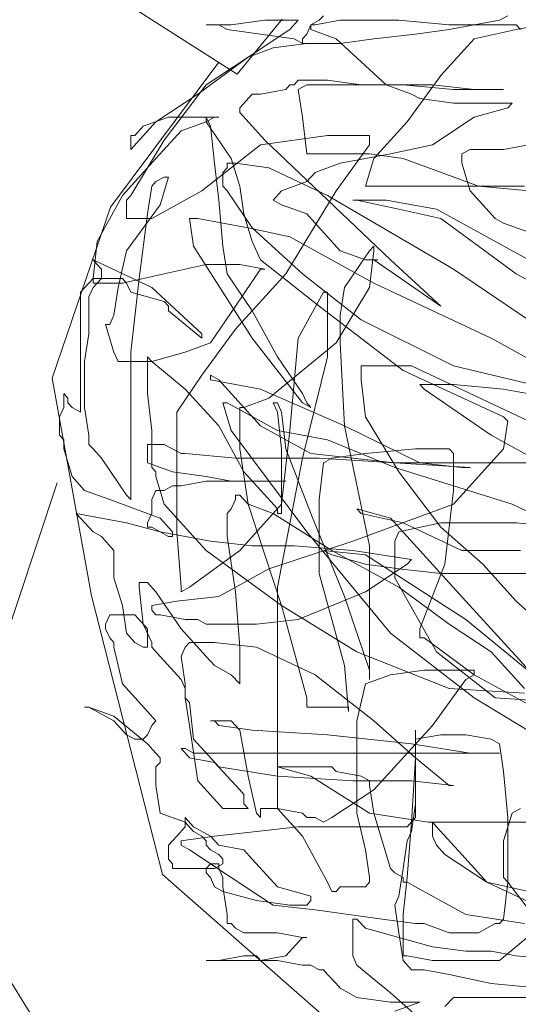
# Model space of a CAD drawing. Units: inches. Extents: x 1994 to 3075, y 3517 to 3950.
# Tile 40 of 58: x 1994.64257 to 1994.646332, y 3553.741889 to 3553.749313. Entities that reach past the tile are written whole.
import ezdxf

# ---------------------------------------------------------------- set-up
doc = ezdxf.new("R2010")
doc.units = ezdxf.units.IN
doc.layers.add('A-FURN-REFR', color=8, linetype='Continuous', lineweight=13)

msp = doc.modelspace()

# ---------------------------------------------------------------- linework, layer by layer
at = {"layer": 'A-FURN-REFR'}
for p, q in [((1994.6422829, 3553.7501317), (1994.644212, 3553.7489025)), ((1994.6444196, 3553.7493078), (1994.6441668, 3553.7492731)), ((1994.644212, 3553.7489025), (1994.644551, 3553.7493173)), ((1994.6446725, 3553.7493078), (1994.6444196, 3553.7493078)), ((1994.6446093, 3553.7492383), (1994.6446725, 3553.7493078)), ((1994.6448306, 3553.7493078), (1994.6447673, 3553.7492731)), ((1994.644799, 3553.7492731), (1994.6449886, 3553.7493078)), ((1994.6448622, 3553.7493426), (1994.6448306, 3553.7493078)), ((1994.6449886, 3553.7493078), (1994.6454312, 3553.7493078)), ((1994.6454312, 3553.7493078), (1994.6458105, 3553.7492731)), ((1994.6460001, 3553.7492731), (1994.6461898, 3553.7493078)), ((1994.6461898, 3553.7493078), (1994.646253, 3553.7493426)), ((1994.6439771, 3553.7492731), (1994.6440719, 3553.7492731)), ((1994.6441668, 3553.7492731), (1994.6439771, 3553.7492731)), ((1994.6440719, 3553.7492731), (1994.6441351, 3553.7492383)), ((1994.6441351, 3553.7492383), (1994.644388, 3553.7492037)), ((1994.6442932, 3553.7490299), (1994.6446093, 3553.7492383)), ((1994.6447673, 3553.7492731), (1994.6447357, 3553.7492037)), ((1994.6447673, 3553.7492731), (1994.644799, 3553.7492731)), ((1994.6447673, 3553.7492383), (1994.6447673, 3553.7492731)), ((1994.644957, 3553.7491689), (1994.6447673, 3553.7492383)), ((1994.6455576, 3553.7492037), (1994.6458105, 3553.7492383)), ((1994.6458105, 3553.7492731), (1994.6463162, 3553.7492731)), ((1994.6458105, 3553.7492383), (1994.6460001, 3553.7492731)), ((1994.6463162, 3553.7492383), (1994.6460001, 3553.7491689)), ((1994.6463162, 3553.7492731), (1994.6463478, 3553.7492383)), ((1994.6465059, 3553.7492731), (1994.6463162, 3553.7492383)), ((1994.644388, 3553.7492037), (1994.6446409, 3553.7491689)), ((1994.6446409, 3553.7491689), (1994.6447041, 3553.7491341)), ((1994.6447357, 3553.7492037), (1994.6447041, 3553.7491689)), ((1994.6447041, 3553.7491689), (1994.6447041, 3553.7491341)), ((1994.6453363, 3553.7488214), (1994.644957, 3553.7491689)), ((1994.6449886, 3553.7491341), (1994.6452415, 3553.7491689)), ((1994.6452415, 3553.7491689), (1994.6455576, 3553.7492037)), ((1994.6460001, 3553.7491689), (1994.6457472, 3553.7488909)), ((1994.6444829, 3553.7490994), (1994.6442932, 3553.7490299)), ((1994.6447357, 3553.7491341), (1994.6444829, 3553.7490994)), ((1994.6447041, 3553.7491341), (1994.6449886, 3553.7491341)), ((1994.6447041, 3553.7491341), (1994.6447357, 3553.7491341)), ((1994.6439139, 3553.7487519), (1994.6442932, 3553.7490299)), ((1994.6442932, 3553.7490299), (1994.6439771, 3553.7488214)), ((1994.6432553, 3553.7478986), (1994.6440722, 3553.7489916)), ((1994.6457472, 3553.7488909), (1994.6454944, 3553.7485434)), ((1994.6439771, 3553.7488214), (1994.643661, 3553.7484045)), ((1994.6445777, 3553.7487867), (1994.644388, 3553.7487519)), ((1994.6446093, 3553.7488214), (1994.6445777, 3553.7487867)), ((1994.6446409, 3553.7488214), (1994.6446093, 3553.7488214)), ((1994.6446725, 3553.7488562), (1994.6446409, 3553.7488214)), ((1994.6448938, 3553.7488562), (1994.6446725, 3553.7488562)), ((1994.6446725, 3553.7487867), (1994.6447357, 3553.7488214)), ((1994.6447041, 3553.7485782), (1994.6446725, 3553.7487867)), ((1994.6447357, 3553.7488214), (1994.645684, 3553.7488214)), ((1994.6451466, 3553.7488214), (1994.6448938, 3553.7488562)), ((1994.6454628, 3553.7488214), (1994.6451466, 3553.7488214)), ((1994.645526, 3553.7487519), (1994.6453363, 3553.7488214)), ((1994.6458421, 3553.7487867), (1994.6454628, 3553.7488214)), ((1994.645684, 3553.7488214), (1994.6460001, 3553.7487867)), ((1994.6462214, 3553.7487867), (1994.6458421, 3553.7487867)), ((1994.6460001, 3553.7487867), (1994.6462214, 3553.7487867)), ((1994.6435978, 3553.7485434), (1994.6439139, 3553.7487519)), ((1994.6443248, 3553.7487519), (1994.64423, 3553.7486477)), ((1994.644388, 3553.7487519), (1994.6443248, 3553.7487519)), ((1994.6455892, 3553.7487172), (1994.645526, 3553.7487519)), ((1994.6458421, 3553.7486824), (1994.6455892, 3553.7487172)), ((1994.64423, 3553.7486477), (1994.64423, 3553.7486129)), ((1994.6462846, 3553.7486824), (1994.6458421, 3553.7486824)), ((1994.6460001, 3553.7485782), (1994.646253, 3553.7486477)), ((1994.646253, 3553.7486477), (1994.6462846, 3553.7486824)), ((1994.6436926, 3553.7485782), (1994.6435029, 3553.7485087)), ((1994.6440719, 3553.7485782), (1994.6436926, 3553.7485782)), ((1994.6439771, 3553.7485782), (1994.6440087, 3553.7485087)), ((1994.6439771, 3553.7485434), (1994.6439771, 3553.7485782)), ((1994.6439771, 3553.7485434), (1994.6440403, 3553.7485782)), ((1994.6440403, 3553.7485782), (1994.6440719, 3553.7485782)), ((1994.64423, 3553.7486129), (1994.6444196, 3553.7484045)), ((1994.6447357, 3553.7483002), (1994.6447041, 3553.7485782)), ((1994.645684, 3553.7483697), (1994.6460001, 3553.7485782)), ((1994.6434081, 3553.7483349), (1994.6435978, 3553.7485434)), ((1994.6435029, 3553.7485087), (1994.6434397, 3553.7484392)), ((1994.6437875, 3553.748474), (1994.6439771, 3553.7485434)), ((1994.6441668, 3553.7482654), (1994.6439771, 3553.7485434)), ((1994.6440087, 3553.7485087), (1994.6440403, 3553.7482307)), ((1994.6454944, 3553.7485434), (1994.6452415, 3553.7482654)), ((1994.6434081, 3553.7484392), (1994.6434081, 3553.7483349)), ((1994.6434397, 3553.7484392), (1994.6434081, 3553.7484392)), ((1994.6435978, 3553.7482654), (1994.6437875, 3553.748474)), ((1994.644388, 3553.7483697), (1994.6448938, 3553.7484392)), ((1994.6448938, 3553.7484392), (1994.6452099, 3553.7484392)), ((1994.6452099, 3553.7484392), (1994.6452099, 3553.7483697)), ((1994.643661, 3553.7484045), (1994.6434081, 3553.7479875)), ((1994.6439455, 3553.7480222), (1994.644388, 3553.7483697)), ((1994.6444196, 3553.7484045), (1994.6453679, 3553.747501)), ((1994.6452099, 3553.7483697), (1994.644957, 3553.7480222)), ((1994.6453679, 3553.7483002), (1994.645684, 3553.7483697)), ((1994.6464111, 3553.7483697), (1994.6462214, 3553.7483349)), ((1994.6452099, 3553.7483002), (1994.6447357, 3553.7483002)), ((1994.6451783, 3553.7482654), (1994.6453679, 3553.7483002)), ((1994.6454628, 3553.7482654), (1994.6452099, 3553.7483002)), ((1994.6459685, 3553.7483349), (1994.6459053, 3553.7483002)), ((1994.6459053, 3553.7483002), (1994.6459053, 3553.7482307)), ((1994.6462214, 3553.7483349), (1994.6459685, 3553.7483349)), ((1994.6433449, 3553.7479875), (1994.6435978, 3553.7482654)), ((1994.6440403, 3553.7482307), (1994.6440719, 3553.7479527)), ((1994.6441035, 3553.7481612), (1994.6441351, 3553.7481959)), ((1994.6441351, 3553.7482307), (1994.6441984, 3553.7482307)), ((1994.6441351, 3553.7481959), (1994.6441351, 3553.7482307)), ((1994.64423, 3553.748057), (1994.6441668, 3553.7482654)), ((1994.6441984, 3553.7482307), (1994.6444512, 3553.7481959)), ((1994.6444512, 3553.7481959), (1994.6448938, 3553.7479875)), ((1994.644799, 3553.7481612), (1994.6449886, 3553.7482307)), ((1994.6449886, 3553.7482307), (1994.6451783, 3553.7482654)), ((1994.6452415, 3553.7482654), (1994.6451783, 3553.748057)), ((1994.6460317, 3553.748057), (1994.6454628, 3553.7482654)), ((1994.6459053, 3553.7482307), (1994.6459685, 3553.7480222)), ((1994.6435978, 3553.7480917), (1994.643661, 3553.7481265)), ((1994.6436926, 3553.7481265), (1994.6436294, 3553.747918)), ((1994.643661, 3553.7481265), (1994.6436926, 3553.7481265)), ((1994.6441035, 3553.748057), (1994.6441035, 3553.7481612)), ((1994.6447357, 3553.7480917), (1994.644799, 3553.7481612)), ((1994.6435346, 3553.7478485), (1994.6435662, 3553.748057)), ((1994.6435662, 3553.748057), (1994.6435978, 3553.7480917)), ((1994.6441351, 3553.7480222), (1994.6441035, 3553.748057)), ((1994.6442616, 3553.7478485), (1994.64423, 3553.748057)), ((1994.6445461, 3553.7480222), (1994.6447357, 3553.7480917)), ((1994.6451783, 3553.748057), (1994.6463794, 3553.748057)), ((1994.6467904, 3553.7479875), (1994.6460317, 3553.748057)), ((1994.6431553, 3553.74764), (1994.6433449, 3553.7479875)), ((1994.6434081, 3553.7479875), (1994.6433765, 3553.7479527)), ((1994.6435662, 3553.7478137), (1994.6439455, 3553.7480222)), ((1994.6443248, 3553.7477443), (1994.6441351, 3553.7480222)), ((1994.6444829, 3553.7479527), (1994.6445461, 3553.7480222)), ((1994.644957, 3553.7480222), (1994.6445777, 3553.7473968)), ((1994.6448938, 3553.7479875), (1994.6458421, 3553.7474316)), ((1994.6459685, 3553.7480222), (1994.6461582, 3553.7478137)), ((1994.6428157, 3553.7466092), (1994.6432553, 3553.7478986)), ((1994.6433765, 3553.7479527), (1994.6433765, 3553.7478137)), ((1994.6436294, 3553.747918), (1994.6433765, 3553.7475705)), ((1994.6440719, 3553.7479527), (1994.6441035, 3553.7476053)), ((1994.6445461, 3553.747918), (1994.6444829, 3553.7479527)), ((1994.6447357, 3553.7478485), (1994.6445461, 3553.747918)), ((1994.6450834, 3553.7479527), (1994.6453363, 3553.7479527)), ((1994.645115, 3553.7479527), (1994.6450834, 3553.7479527)), ((1994.6454312, 3553.7478832), (1994.645115, 3553.7479527)), ((1994.6453363, 3553.7479527), (1994.6457156, 3553.7478832)), ((1994.6434713, 3553.747362), (1994.6435346, 3553.7478485)), ((1994.6443248, 3553.74764), (1994.6442616, 3553.7478485)), ((1994.644799, 3553.747779), (1994.6447357, 3553.7478485)), ((1994.6457472, 3553.7478137), (1994.6454312, 3553.7478832)), ((1994.6457156, 3553.7478832), (1994.6464743, 3553.7474662)), ((1994.6433765, 3553.7478137), (1994.6435662, 3553.7478137)), ((1994.6438507, 3553.7478137), (1994.6439139, 3553.7478137)), ((1994.6438823, 3553.7476053), (1994.6438507, 3553.7478137)), ((1994.6439139, 3553.7478137), (1994.6441035, 3553.747779)), ((1994.6441035, 3553.747779), (1994.6442932, 3553.7477443)), ((1994.6449886, 3553.7475705), (1994.644799, 3553.747779)), ((1994.6463162, 3553.7473968), (1994.6457472, 3553.7478137)), ((1994.6461582, 3553.7478137), (1994.6462214, 3553.747779)), ((1994.6462214, 3553.747779), (1994.6464111, 3553.7477095)), ((1994.6442932, 3553.7477443), (1994.6446093, 3553.7476748)), ((1994.6447041, 3553.7473968), (1994.6443248, 3553.7477443)), ((1994.6446093, 3553.7476748), (1994.6452415, 3553.7473273)), ((1994.6431236, 3553.747362), (1994.6431553, 3553.74764)), ((1994.6443248, 3553.7469103), (1994.6438823, 3553.7476053)), ((1994.6441035, 3553.7476053), (1994.6441351, 3553.7473968)), ((1994.644388, 3553.747501), (1994.6443248, 3553.74764)), ((1994.6452099, 3553.7475705), (1994.6452415, 3553.7476053)), ((1994.6452415, 3553.7476053), (1994.6452415, 3553.7475705)), ((1994.6433765, 3553.7475705), (1994.6433133, 3553.7472925)), ((1994.6451783, 3553.747501), (1994.6449886, 3553.7475705)), ((1994.6450202, 3553.7472925), (1994.6452099, 3553.7475705)), ((1994.6452415, 3553.7475705), (1994.6452099, 3553.7472925)), ((1994.6431236, 3553.747501), (1994.6435662, 3553.7472925)), ((1994.6431553, 3553.7474662), (1994.6431236, 3553.747501)), ((1994.6431869, 3553.7474316), (1994.6431553, 3553.7474662)), ((1994.6439771, 3553.7474662), (1994.643661, 3553.7473968)), ((1994.64423, 3553.7474662), (1994.6439771, 3553.7474662)), ((1994.6444196, 3553.7474316), (1994.64423, 3553.7474662)), ((1994.6448306, 3553.7471535), (1994.644388, 3553.747501)), ((1994.6452731, 3553.747501), (1994.6451783, 3553.747501)), ((1994.6452415, 3553.747501), (1994.6452731, 3553.747501)), ((1994.6457472, 3553.7471535), (1994.6452415, 3553.747501)), ((1994.6453679, 3553.747501), (1994.6457472, 3553.7471535)), ((1994.6431869, 3553.747362), (1994.6431869, 3553.7474316)), ((1994.643661, 3553.7473968), (1994.6433449, 3553.7473273)), ((1994.6441351, 3553.7473968), (1994.6443248, 3553.7471188)), ((1994.6441984, 3553.7471535), (1994.644388, 3553.7474316)), ((1994.6445777, 3553.7473968), (1994.6441984, 3553.7469798)), ((1994.644388, 3553.7474316), (1994.6444196, 3553.7474316)), ((1994.6451466, 3553.7470493), (1994.6447041, 3553.7473968)), ((1994.6458421, 3553.7474316), (1994.6466639, 3553.7468756)), ((1994.6469484, 3553.7470493), (1994.6463162, 3553.7473968)), ((1994.6430288, 3553.7472578), (1994.6431236, 3553.747362)), ((1994.6431236, 3553.7473273), (1994.6431236, 3553.747362)), ((1994.6431869, 3553.747362), (1994.6431236, 3553.7472925)), ((1994.6431236, 3553.747362), (1994.6431869, 3553.747362)), ((1994.6433449, 3553.7473273), (1994.6431236, 3553.7473273)), ((1994.6433449, 3553.747362), (1994.6431869, 3553.747362)), ((1994.6433765, 3553.7473273), (1994.6433449, 3553.747362)), ((1994.6434081, 3553.7472578), (1994.6433765, 3553.7473273)), ((1994.6434081, 3553.7468061), (1994.6434713, 3553.747362)), ((1994.6452415, 3553.7473273), (1994.6461265, 3553.7469103)), ((1994.6430288, 3553.7463544), (1994.6430288, 3553.7472578)), ((1994.6431236, 3553.7472925), (1994.643092, 3553.747223)), ((1994.6433133, 3553.7472925), (1994.6432817, 3553.747084)), ((1994.643661, 3553.7471883), (1994.6434081, 3553.7472578)), ((1994.6435662, 3553.7472925), (1994.6439455, 3553.7469451)), ((1994.6446725, 3553.7469103), (1994.6448622, 3553.7472578)), ((1994.6448622, 3553.7472578), (1994.6448938, 3553.7472578)), ((1994.6448938, 3553.7472578), (1994.6448938, 3553.7467713)), ((1994.6452099, 3553.7472925), (1994.644957, 3553.7468756)), ((1994.6449886, 3553.747084), (1994.6450202, 3553.7472925)), ((1994.643092, 3553.747223), (1994.643092, 3553.7469451)), ((1994.6436926, 3553.7471535), (1994.643661, 3553.7471883)), ((1994.6436926, 3553.7471188), (1994.6436926, 3553.7471535)), ((1994.6440087, 3553.7468756), (1994.6441984, 3553.7471535)), ((1994.6454628, 3553.7466671), (1994.6448306, 3553.7471535)), ((1994.6432817, 3553.747084), (1994.6432501, 3553.7470146)), ((1994.6439455, 3553.7469103), (1994.6436926, 3553.7471188)), ((1994.6443248, 3553.7471188), (1994.6445145, 3553.7467713)), ((1994.6449886, 3553.7468756), (1994.6449886, 3553.747084)), ((1994.6432185, 3553.7470146), (1994.6432817, 3553.7468061)), ((1994.6432501, 3553.7470146), (1994.6432185, 3553.7470146)), ((1994.6458421, 3553.7467019), (1994.6451466, 3553.7470493)), ((1994.643092, 3553.7469451), (1994.6430604, 3553.7467365)), ((1994.6441984, 3553.7469798), (1994.6439455, 3553.7466324)), ((1994.6439455, 3553.7469451), (1994.6439455, 3553.7469103)), ((1994.6438191, 3553.7468061), (1994.6440087, 3553.7468756)), ((1994.6447041, 3553.7464238), (1994.6443248, 3553.7469103)), ((1994.644957, 3553.7468756), (1994.6444512, 3553.7464586)), ((1994.6446093, 3553.7462154), (1994.6446725, 3553.7469103)), ((1994.6450202, 3553.7462501), (1994.6449886, 3553.7468756)), ((1994.6461265, 3553.7469103), (1994.6472645, 3553.7462849)), ((1994.6432817, 3553.7468061), (1994.6433133, 3553.7467365)), ((1994.6434081, 3553.7456941), (1994.6434081, 3553.7468061)), ((1994.6435662, 3553.7467365), (1994.6438191, 3553.7468061)), ((1994.6430604, 3553.7467365), (1994.6430604, 3553.7463891)), ((1994.6433133, 3553.7467365), (1994.6435662, 3553.7467365)), ((1994.6435346, 3553.7467713), (1994.6435662, 3553.7467365)), ((1994.6435346, 3553.7464933), (1994.6435346, 3553.7467713)), ((1994.6435662, 3553.7467365), (1994.6438191, 3553.7465281)), ((1994.6445145, 3553.7467713), (1994.6447041, 3553.7464933)), ((1994.6448938, 3553.7467713), (1994.6447041, 3553.7460069)), ((1994.6451466, 3553.7467019), (1994.645526, 3553.7467019)), ((1994.6451466, 3553.7465976), (1994.6451466, 3553.7467019)), ((1994.6462214, 3553.7463196), (1994.6454628, 3553.7466671)), ((1994.645526, 3553.7467019), (1994.6459685, 3553.7464933)), ((1994.6467271, 3553.7464933), (1994.6458421, 3553.7467019)), ((1994.6431121, 3553.7449681), (1994.6428157, 3553.7466092)), ((1994.6439455, 3553.7466324), (1994.6437558, 3553.7463544)), ((1994.6440087, 3553.7466324), (1994.6440087, 3553.7465976)), ((1994.6440719, 3553.7465976), (1994.6440087, 3553.7466324)), ((1994.6440087, 3553.7465976), (1994.644388, 3553.7465281)), ((1994.644388, 3553.7462501), (1994.6440719, 3553.7465976)), ((1994.6451783, 3553.7463196), (1994.6451466, 3553.7465976)), ((1994.6455892, 3553.7465628), (1994.6456208, 3553.7465281)), ((1994.6458421, 3553.7465628), (1994.6455892, 3553.7465628)), ((1994.6462214, 3553.7465281), (1994.6458421, 3553.7465628)), ((1994.6429024, 3553.7464933), (1994.642934, 3553.7464586)), ((1994.6429024, 3553.7463891), (1994.6429024, 3553.7464933)), ((1994.6435662, 3553.7462154), (1994.6435346, 3553.7464933)), ((1994.6438191, 3553.7465281), (1994.6440719, 3553.7462501)), ((1994.644388, 3553.7465281), (1994.6450202, 3553.7462501)), ((1994.6447041, 3553.7464933), (1994.6447357, 3553.7464238)), ((1994.6456208, 3553.7465281), (1994.6461265, 3553.7461806)), ((1994.6459685, 3553.7464933), (1994.6464111, 3553.7462849)), ((1994.6466007, 3553.7464586), (1994.6462214, 3553.7465281)), ((1994.642934, 3553.7464586), (1994.642934, 3553.7464238)), ((1994.642934, 3553.7464238), (1994.6429656, 3553.7463891)), ((1994.6441035, 3553.7464238), (1994.6441351, 3553.7464238)), ((1994.6441668, 3553.7462154), (1994.6441035, 3553.7464238)), ((1994.6441351, 3553.7464238), (1994.6445145, 3553.7462154)), ((1994.6444512, 3553.7464586), (1994.6442616, 3553.7463891)), ((1994.6444829, 3553.7464238), (1994.6445145, 3553.7464238)), ((1994.6445145, 3553.7463544), (1994.6444829, 3553.7464238)), ((1994.6445145, 3553.7464238), (1994.6445461, 3553.7463544)), ((1994.6447673, 3553.7463891), (1994.6447041, 3553.7464238)), ((1994.6447357, 3553.7464238), (1994.6447673, 3553.7463891)), ((1994.6428708, 3553.7463196), (1994.6429024, 3553.7463891)), ((1994.6429656, 3553.7463891), (1994.6430288, 3553.7463544)), ((1994.6430604, 3553.7463891), (1994.643092, 3553.7461806)), ((1994.6437558, 3553.7463544), (1994.6437558, 3553.7454509)), ((1994.64423, 3553.7463891), (1994.64423, 3553.7460764)), ((1994.6442616, 3553.7463891), (1994.64423, 3553.7463891)), ((1994.6445461, 3553.7460764), (1994.6445145, 3553.7463544)), ((1994.6445461, 3553.7463544), (1994.6445777, 3553.7460764)), ((1994.6428708, 3553.7461806), (1994.6428708, 3553.7463196)), ((1994.6454312, 3553.7459027), (1994.6451783, 3553.7463196)), ((1994.646253, 3553.7462849), (1994.6462214, 3553.7463196)), ((1994.6462214, 3553.7460764), (1994.646253, 3553.7462849)), ((1994.6435662, 3553.7459374), (1994.6435662, 3553.7462154)), ((1994.6440719, 3553.7462501), (1994.6442616, 3553.7459027)), ((1994.6447357, 3553.7454509), (1994.6441668, 3553.7462154)), ((1994.6447673, 3553.7460416), (1994.644388, 3553.7462501)), ((1994.6445145, 3553.7462154), (1994.6448938, 3553.7461459)), ((1994.6445461, 3553.7456594), (1994.6446093, 3553.7462154)), ((1994.6450202, 3553.7462501), (1994.6455892, 3553.7459722)), ((1994.6452099, 3553.7453467), (1994.6450202, 3553.7462501)), ((1994.6429024, 3553.7461459), (1994.6428708, 3553.7461806)), ((1994.6429024, 3553.7460764), (1994.6429024, 3553.7461459)), ((1994.643092, 3553.7461806), (1994.643092, 3553.7461111)), ((1994.6448938, 3553.7461459), (1994.6453996, 3553.7459374)), ((1994.6461265, 3553.7461806), (1994.6466323, 3553.7459027)), ((1994.6429656, 3553.7458679), (1994.6429024, 3553.7460764)), ((1994.643092, 3553.7461111), (1994.6431236, 3553.7460764)), ((1994.6431236, 3553.7460764), (1994.6431869, 3553.7460069)), ((1994.6435346, 3553.7461111), (1994.6435346, 3553.7459722)), ((1994.643661, 3553.7461111), (1994.6435346, 3553.7461111)), ((1994.6437875, 3553.7460416), (1994.643661, 3553.7461111)), ((1994.6438191, 3553.7460416), (1994.6437875, 3553.7460416)), ((1994.6441984, 3553.7460069), (1994.6438191, 3553.7460416)), ((1994.64423, 3553.7460764), (1994.6442932, 3553.7456594)), ((1994.6445461, 3553.7455899), (1994.6445461, 3553.7460764)), ((1994.6445777, 3553.7460764), (1994.6447673, 3553.7455899)), ((1994.6453996, 3553.7459722), (1994.6447673, 3553.7460416)), ((1994.6449254, 3553.7460069), (1994.6451783, 3553.7460416)), ((1994.6451783, 3553.7460416), (1994.6455576, 3553.7460764)), ((1994.6455576, 3553.7460764), (1994.6458105, 3553.7460764)), ((1994.6458105, 3553.7460764), (1994.6458421, 3553.7460416)), ((1994.6458421, 3553.7456594), (1994.6462214, 3553.7460764)), ((1994.6458421, 3553.7460416), (1994.6458421, 3553.7457636)), ((1994.6431869, 3553.7460069), (1994.6433765, 3553.7457289)), ((1994.6435346, 3553.7459722), (1994.6437242, 3553.7459027)), ((1994.6448306, 3553.7460069), (1994.6441984, 3553.7460069)), ((1994.6447041, 3553.7460069), (1994.6445145, 3553.745034)), ((1994.6453996, 3553.7459722), (1994.6448306, 3553.7460069)), ((1994.6448306, 3553.7456941), (1994.6448622, 3553.7459722)), ((1994.6448622, 3553.7459722), (1994.6449254, 3553.7460069)), ((1994.6459685, 3553.7459374), (1994.6453996, 3553.7459722)), ((1994.6468536, 3553.7459722), (1994.6453996, 3553.7459722)), ((1994.6455892, 3553.7459722), (1994.6459053, 3553.7459374)), ((1994.6435978, 3553.7459027), (1994.6435662, 3553.7459374)), ((1994.6435978, 3553.7458679), (1994.6435978, 3553.7459027)), ((1994.6437242, 3553.7459027), (1994.6439771, 3553.7458679)), ((1994.6442616, 3553.7459027), (1994.6445145, 3553.7456247)), ((1994.6453996, 3553.7459374), (1994.6462846, 3553.7456594)), ((1994.6457472, 3553.7454857), (1994.6454312, 3553.7459027)), ((1994.6459053, 3553.7459374), (1994.6459685, 3553.7459374)), ((1994.6428544, 3553.7458217), (1994.6419152, 3553.7430024)), ((1994.6430604, 3553.7457636), (1994.6429656, 3553.7458679)), ((1994.643661, 3553.7456594), (1994.6435978, 3553.7458679)), ((1994.6439771, 3553.7458332), (1994.6437875, 3553.7457984)), ((1994.6439771, 3553.7458679), (1994.6441668, 3553.7458332)), ((1994.6445777, 3553.7458332), (1994.6439771, 3553.7458332)), ((1994.6441668, 3553.7458332), (1994.6445777, 3553.7458332)), ((1994.6432501, 3553.7456941), (1994.6430604, 3553.7457636)), ((1994.6435978, 3553.7457636), (1994.6435662, 3553.7456941)), ((1994.643661, 3553.7457636), (1994.6435978, 3553.7457636)), ((1994.6437242, 3553.7457984), (1994.643661, 3553.7457636)), ((1994.6437875, 3553.7457984), (1994.6437242, 3553.7457984)), ((1994.6458421, 3553.7457636), (1994.6457789, 3553.7452077)), ((1994.6434397, 3553.7456247), (1994.6432501, 3553.7456941)), ((1994.6433765, 3553.7457289), (1994.6434081, 3553.7456941)), ((1994.6435662, 3553.7456941), (1994.6435662, 3553.7455899)), ((1994.6441668, 3553.7456247), (1994.6441984, 3553.7456941)), ((1994.6441984, 3553.7457289), (1994.64423, 3553.7457289)), ((1994.6441984, 3553.7456941), (1994.6441984, 3553.7457289)), ((1994.64423, 3553.7457289), (1994.6442932, 3553.7456594)), ((1994.6448306, 3553.7451382), (1994.6448306, 3553.7456941)), ((1994.6436294, 3553.7455552), (1994.6434397, 3553.7456247)), ((1994.6439771, 3553.7453119), (1994.643661, 3553.7456594)), ((1994.6441351, 3553.7455899), (1994.6441668, 3553.7456247)), ((1994.64423, 3553.7453119), (1994.6445461, 3553.7456594)), ((1994.6442932, 3553.7456594), (1994.6445461, 3553.744895)), ((1994.6442932, 3553.7456594), (1994.6444829, 3553.7455899)), ((1994.6445145, 3553.7456247), (1994.6445145, 3553.7455899)), ((1994.6450834, 3553.7453814), (1994.6458421, 3553.7456594)), ((1994.645115, 3553.7456247), (1994.6453679, 3553.7455552)), ((1994.6451466, 3553.7455899), (1994.645115, 3553.7456247)), ((1994.6462846, 3553.7456594), (1994.6471697, 3553.7452425)), ((1994.6429972, 3553.7455899), (1994.6433765, 3553.7455204)), ((1994.6431236, 3553.7454509), (1994.6429972, 3553.7455899)), ((1994.6433765, 3553.7455204), (1994.6436294, 3553.7454509)), ((1994.6435662, 3553.7455899), (1994.6435346, 3553.7455204)), ((1994.6435346, 3553.7455204), (1994.6435346, 3553.7454857)), ((1994.6437242, 3553.7454509), (1994.6436294, 3553.7455552)), ((1994.6441351, 3553.7454162), (1994.6441351, 3553.7455899)), ((1994.6444829, 3553.7455899), (1994.6449254, 3553.7453119)), ((1994.6445145, 3553.7455899), (1994.6445461, 3553.7455899)), ((1994.6447673, 3553.7455899), (1994.6450202, 3553.7449644)), ((1994.6454628, 3553.7455204), (1994.6451466, 3553.7455899)), ((1994.6453679, 3553.7455552), (1994.6459369, 3553.7449298)), ((1994.6454312, 3553.7454509), (1994.6457472, 3553.7455204)), ((1994.6459053, 3553.7453119), (1994.6454628, 3553.7455204)), ((1994.6457472, 3553.7455204), (1994.6463162, 3553.7455204)), ((1994.6463162, 3553.7455204), (1994.6470116, 3553.7454509)), ((1994.6431869, 3553.7454162), (1994.6431236, 3553.7454509)), ((1994.6435346, 3553.7454857), (1994.6435662, 3553.7454857)), ((1994.6435662, 3553.7454857), (1994.6436294, 3553.7454509)), ((1994.6436294, 3553.7454509), (1994.6440087, 3553.7453814)), ((1994.6436294, 3553.7454509), (1994.6436926, 3553.7454162)), ((1994.6437242, 3553.7454162), (1994.6437242, 3553.7454509)), ((1994.6437558, 3553.7454509), (1994.6437875, 3553.745034)), ((1994.6453679, 3553.7446865), (1994.6447357, 3553.7454509)), ((1994.6453996, 3553.7453814), (1994.6454312, 3553.7454509)), ((1994.6460633, 3553.7452077), (1994.6457472, 3553.7454857)), ((1994.6432817, 3553.7453119), (1994.6431869, 3553.7454162)), ((1994.6436926, 3553.7454162), (1994.6437242, 3553.7454162)), ((1994.6440087, 3553.7453814), (1994.6443248, 3553.7453467)), ((1994.6441984, 3553.7449992), (1994.6441351, 3553.7454162)), ((1994.6444512, 3553.745173), (1994.6450834, 3553.7453814)), ((1994.6453996, 3553.7451035), (1994.6453996, 3553.7453814)), ((1994.6432817, 3553.7451035), (1994.6432817, 3553.7453119)), ((1994.6438507, 3553.745034), (1994.64423, 3553.7453119)), ((1994.6445461, 3553.744895), (1994.6439771, 3553.7453119)), ((1994.6443248, 3553.7453467), (1994.6446409, 3553.7453467)), ((1994.6446409, 3553.7453467), (1994.6450834, 3553.7453119)), ((1994.6448622, 3553.7453119), (1994.6451783, 3553.7452772)), ((1994.6449254, 3553.7452772), (1994.6448622, 3553.7453119)), ((1994.6449254, 3553.7453119), (1994.6454312, 3553.745034)), ((1994.6450834, 3553.7453119), (1994.645526, 3553.7452425)), ((1994.6452099, 3553.744339), (1994.6452099, 3553.7453467)), ((1994.6463478, 3553.7453119), (1994.6459053, 3553.7453119)), ((1994.6451783, 3553.7452077), (1994.6449254, 3553.7452772)), ((1994.6451783, 3553.7452772), (1994.6459369, 3553.7447907)), ((1994.645526, 3553.7452425), (1994.6454944, 3553.7452077)), ((1994.6440719, 3553.7449644), (1994.6444512, 3553.745173)), ((1994.6454944, 3553.7452077), (1994.6451783, 3553.7449992)), ((1994.6454312, 3553.745173), (1994.6451783, 3553.7452077)), ((1994.6457472, 3553.7451382), (1994.6454312, 3553.745173)), ((1994.6457789, 3553.7452077), (1994.6455892, 3553.7447212)), ((1994.6463162, 3553.7449298), (1994.6460633, 3553.7452077)), ((1994.6433449, 3553.744895), (1994.6432817, 3553.7451035)), ((1994.6450202, 3553.7444433), (1994.6448306, 3553.7451382)), ((1994.6457156, 3553.7445475), (1994.6453996, 3553.7451035)), ((1994.6466323, 3553.7451382), (1994.6457472, 3553.7451382)), ((1994.6434713, 3553.7450687), (1994.6435346, 3553.7450687)), ((1994.6434713, 3553.745034), (1994.6434713, 3553.7450687)), ((1994.6435029, 3553.744756), (1994.6434713, 3553.745034)), ((1994.6435346, 3553.7450687), (1994.6435978, 3553.7449992)), ((1994.6437875, 3553.7449992), (1994.6438507, 3553.745034)), ((1994.6437875, 3553.745034), (1994.6437875, 3553.7449992)), ((1994.6445145, 3553.745034), (1994.6445145, 3553.7436788)), ((1994.6454312, 3553.745034), (1994.6458105, 3553.744756)), ((1994.6436467, 3553.7428672), (1994.6431121, 3553.7449681)), ((1994.6435662, 3553.744895), (1994.6437558, 3553.7449298)), ((1994.6435978, 3553.7449992), (1994.6437875, 3553.7447212)), ((1994.6437558, 3553.7449298), (1994.6440719, 3553.7449644)), ((1994.64423, 3553.7445822), (1994.6441984, 3553.7449992)), ((1994.6451783, 3553.7449992), (1994.6446725, 3553.7447907)), ((1994.6450202, 3553.7449644), (1994.6452099, 3553.7444085)), ((1994.6459369, 3553.7449298), (1994.6466323, 3553.7441653)), ((1994.6466955, 3553.7445822), (1994.6463162, 3553.7449298)), ((1994.6433765, 3553.7446865), (1994.6433449, 3553.744895)), ((1994.6435662, 3553.7448603), (1994.6435662, 3553.744895)), ((1994.6435978, 3553.7448255), (1994.6435662, 3553.7448603)), ((1994.6445461, 3553.744895), (1994.6447357, 3553.7442001)), ((1994.645115, 3553.7445475), (1994.6445461, 3553.744895)), ((1994.6432185, 3553.744756), (1994.6432501, 3553.7448255)), ((1994.6432501, 3553.7448255), (1994.6434397, 3553.7448255)), ((1994.6434397, 3553.7448255), (1994.6435346, 3553.7447212)), ((1994.6436294, 3553.7448255), (1994.6435978, 3553.7448255)), ((1994.6438191, 3553.7447907), (1994.6436294, 3553.7448255)), ((1994.6439139, 3553.7447907), (1994.6438191, 3553.7447907)), ((1994.6439771, 3553.744756), (1994.6439139, 3553.7447907)), ((1994.6446725, 3553.7447907), (1994.6443564, 3553.744756)), ((1994.6459369, 3553.7447907), (1994.6466955, 3553.7441653)), ((1994.6432185, 3553.7447212), (1994.6432185, 3553.744756)), ((1994.6432501, 3553.7446517), (1994.6432185, 3553.7447212)), ((1994.6435662, 3553.744617), (1994.6435029, 3553.744756)), ((1994.6435346, 3553.7447212), (1994.6435346, 3553.7445822)), ((1994.6437875, 3553.7447212), (1994.6439771, 3553.7445128)), ((1994.6443564, 3553.744756), (1994.6439771, 3553.744756)), ((1994.6455892, 3553.7447212), (1994.6455892, 3553.7446517)), ((1994.6458105, 3553.744756), (1994.6461265, 3553.7445475)), ((1994.6432817, 3553.744617), (1994.6432501, 3553.7446517)), ((1994.6434397, 3553.744617), (1994.6433765, 3553.7446865)), ((1994.6460001, 3553.7442001), (1994.6453679, 3553.7446865)), ((1994.6455892, 3553.7446517), (1994.6456208, 3553.7446517)), ((1994.6456208, 3553.7446517), (1994.6460001, 3553.7443738)), ((1994.6432817, 3553.7445822), (1994.6432817, 3553.744617)), ((1994.6433449, 3553.7443043), (1994.6432817, 3553.7445822)), ((1994.6435029, 3553.7445822), (1994.6434397, 3553.744617)), ((1994.6435346, 3553.7445822), (1994.6435029, 3553.7445822)), ((1994.6435662, 3553.7445822), (1994.6435662, 3553.744617)), ((1994.6436294, 3553.7445128), (1994.6435662, 3553.7445822)), ((1994.6437875, 3553.7445128), (1994.6438191, 3553.7445822)), ((1994.6438191, 3553.7445822), (1994.6438507, 3553.744617)), ((1994.6438507, 3553.744617), (1994.6440403, 3553.744617)), ((1994.6440403, 3553.744617), (1994.6443564, 3553.7445822)), ((1994.64423, 3553.7443043), (1994.64423, 3553.7445822)), ((1994.6443564, 3553.7445822), (1994.644799, 3553.7443738)), ((1994.6437875, 3553.744339), (1994.6436294, 3553.7445128)), ((1994.6438191, 3553.7443043), (1994.6437875, 3553.7445128)), ((1994.6439771, 3553.7445128), (1994.6440403, 3553.7444433)), ((1994.6458105, 3553.7442695), (1994.645115, 3553.7445475)), ((1994.6461582, 3553.7442001), (1994.6457156, 3553.7445475)), ((1994.6461265, 3553.7445475), (1994.6463794, 3553.7442695)), ((1994.6440403, 3553.7444433), (1994.6441668, 3553.7443738)), ((1994.6450518, 3553.7440958), (1994.6450202, 3553.7444433)), ((1994.6452099, 3553.7444085), (1994.6452099, 3553.744339)), ((1994.6453679, 3553.7443738), (1994.6456208, 3553.7444085)), ((1994.6456208, 3553.7444085), (1994.6460001, 3553.7444085)), ((1994.6460001, 3553.7444085), (1994.6460001, 3553.7443738)), ((1994.6438191, 3553.7442695), (1994.6437875, 3553.744339)), ((1994.6441668, 3553.7443738), (1994.64423, 3553.7443043)), ((1994.644799, 3553.7443738), (1994.6452415, 3553.7440263)), ((1994.6451783, 3553.7443043), (1994.6453679, 3553.7443738)), ((1994.6459369, 3553.744339), (1994.645684, 3553.7439915)), ((1994.6460001, 3553.7443738), (1994.6459369, 3553.744339)), ((1994.6460001, 3553.7443738), (1994.6465059, 3553.7440958)), ((1994.6435346, 3553.7440958), (1994.6433449, 3553.7443043)), ((1994.6438191, 3553.7442001), (1994.6438191, 3553.7443043)), ((1994.6438191, 3553.7442001), (1994.6438191, 3553.7442695)), ((1994.645115, 3553.7440263), (1994.6451783, 3553.7443043)), ((1994.6463794, 3553.7442348), (1994.6458105, 3553.7442695)), ((1994.6438507, 3553.7441653), (1994.6438191, 3553.7442001)), ((1994.6438507, 3553.7439915), (1994.6438191, 3553.7442001)), ((1994.6447357, 3553.7442001), (1994.6447357, 3553.7441306)), ((1994.6465691, 3553.7438526), (1994.6460001, 3553.7442001)), ((1994.6471697, 3553.7441306), (1994.6461582, 3553.7442001)), ((1994.6430604, 3553.7441306), (1994.643092, 3553.7441306)), ((1994.643092, 3553.7441306), (1994.6430604, 3553.7441306)), ((1994.643092, 3553.7441306), (1994.6432817, 3553.7440263)), ((1994.6432817, 3553.7440611), (1994.643092, 3553.7441306)), ((1994.6438823, 3553.7438873), (1994.6438507, 3553.7441653)), ((1994.6447357, 3553.7441306), (1994.6450518, 3553.7441306)), ((1994.6450518, 3553.7441306), (1994.6450518, 3553.7440958)), ((1994.6435346, 3553.7438526), (1994.6432817, 3553.7440611)), ((1994.6435978, 3553.7440263), (1994.6435346, 3553.7440958)), ((1994.6432817, 3553.7440263), (1994.6433765, 3553.743922)), ((1994.6435346, 3553.743922), (1994.6435662, 3553.7439915)), ((1994.6435662, 3553.7439915), (1994.6435978, 3553.7440263)), ((1994.6439139, 3553.7435746), (1994.6438507, 3553.7439915)), ((1994.6440087, 3553.7440263), (1994.6440403, 3553.7440263)), ((1994.6441668, 3553.7440263), (1994.6440087, 3553.7440263)), ((1994.6440403, 3553.7440263), (1994.6440719, 3553.7439915)), ((1994.6440719, 3553.7439915), (1994.6443248, 3553.7439568)), ((1994.64423, 3553.7439568), (1994.6441668, 3553.7440263)), ((1994.645115, 3553.7433314), (1994.645115, 3553.7440263)), ((1994.6452415, 3553.7440263), (1994.6455576, 3553.7437483)), ((1994.645684, 3553.7439915), (1994.6452415, 3553.7435051)), ((1994.6433765, 3553.743922), (1994.6434397, 3553.7438873)), ((1994.6434397, 3553.7438873), (1994.6435029, 3553.7438873)), ((1994.6435029, 3553.7438873), (1994.6435346, 3553.743922)), ((1994.6440719, 3553.7436788), (1994.6438823, 3553.7438873)), ((1994.6442932, 3553.7436093), (1994.64423, 3553.7439568)), ((1994.6443248, 3553.7439568), (1994.6448938, 3553.743922)), ((1994.6448938, 3553.743922), (1994.645526, 3553.7438526)), ((1994.6455576, 3553.7439568), (1994.6455576, 3553.7437483)), ((1994.6455576, 3553.7432966), (1994.6455576, 3553.7439568)), ((1994.6455576, 3553.7438873), (1994.6457472, 3553.743922)), ((1994.6455576, 3553.7434009), (1994.6455576, 3553.7438873)), ((1994.6457472, 3553.743922), (1994.6459369, 3553.743922)), ((1994.6459369, 3553.743922), (1994.6461265, 3553.7438873)), ((1994.6461265, 3553.7438873), (1994.6461898, 3553.7438526)), ((1994.6435978, 3553.7437831), (1994.6435346, 3553.7438526)), ((1994.6437875, 3553.7438178), (1994.6438507, 3553.7437483)), ((1994.6438191, 3553.7438178), (1994.6437875, 3553.7438178)), ((1994.6438823, 3553.7437831), (1994.6438191, 3553.7438178)), ((1994.645526, 3553.7438526), (1994.6459685, 3553.7437831)), ((1994.6461898, 3553.7438526), (1994.6462214, 3553.7436441)), ((1994.6436294, 3553.7437483), (1994.6435978, 3553.7437831)), ((1994.6436294, 3553.7437136), (1994.6436294, 3553.7437483)), ((1994.6438507, 3553.7437483), (1994.6440403, 3553.7437136)), ((1994.6461898, 3553.7437831), (1994.6438823, 3553.7437831)), ((1994.6455576, 3553.7437483), (1994.645526, 3553.7432619)), ((1994.6455576, 3553.7437483), (1994.6458105, 3553.7435398)), ((1994.6459685, 3553.7437831), (1994.6461898, 3553.7437831)), ((1994.6435978, 3553.7436788), (1994.6436294, 3553.7437136)), ((1994.6435978, 3553.7435398), (1994.6435978, 3553.7436788)), ((1994.6440403, 3553.7437136), (1994.64423, 3553.7435051)), ((1994.6445145, 3553.7436093), (1994.6440719, 3553.7436788)), ((1994.6445145, 3553.7436788), (1994.6445145, 3553.7433661)), ((1994.6449254, 3553.7436788), (1994.6445145, 3553.7436788)), ((1994.6445145, 3553.7436788), (1994.6447673, 3553.7436093)), ((1994.644957, 3553.7436441), (1994.6449254, 3553.7436788)), ((1994.6443564, 3553.7433314), (1994.6442932, 3553.7436093)), ((1994.6450834, 3553.7435746), (1994.6445145, 3553.7436093)), ((1994.6447673, 3553.7436093), (1994.6452099, 3553.7433314)), ((1994.6451466, 3553.7436093), (1994.644957, 3553.7436441)), ((1994.6452099, 3553.7435746), (1994.6451466, 3553.7436093)), ((1994.6462214, 3553.7436441), (1994.646253, 3553.7432966)), ((1994.6436294, 3553.7433314), (1994.6435978, 3553.7435398)), ((1994.6441035, 3553.7433661), (1994.6439139, 3553.7435746)), ((1994.645526, 3553.7435746), (1994.6450834, 3553.7435746)), ((1994.6452099, 3553.7435398), (1994.6452099, 3553.7435746)), ((1994.6452415, 3553.7433314), (1994.6452099, 3553.7435398)), ((1994.6458421, 3553.7435398), (1994.645526, 3553.7435746)), ((1994.6458105, 3553.7435398), (1994.6458421, 3553.7435398)), ((1994.64423, 3553.7435051), (1994.6442616, 3553.7434704)), ((1994.6442616, 3553.7434704), (1994.6442616, 3553.7434009)), ((1994.6452415, 3553.7435051), (1994.6449254, 3553.7432966)), ((1994.6442616, 3553.7434009), (1994.6442932, 3553.7433661)), ((1994.645526, 3553.7431923), (1994.6455576, 3553.7434009)), ((1994.6438191, 3553.7432619), (1994.6436294, 3553.7433314)), ((1994.6438191, 3553.7432966), (1994.6438191, 3553.7432271)), ((1994.6438823, 3553.7432271), (1994.6438191, 3553.7432966)), ((1994.6442932, 3553.7433661), (1994.6441035, 3553.7433661)), ((1994.644388, 3553.7432966), (1994.6443564, 3553.7433314)), ((1994.644388, 3553.7433661), (1994.644388, 3553.7432966)), ((1994.6445145, 3553.7433661), (1994.644388, 3553.7433661)), ((1994.6447041, 3553.7433314), (1994.6445145, 3553.7433661)), ((1994.6445145, 3553.7433661), (1994.6447041, 3553.7431576)), ((1994.6447357, 3553.7432966), (1994.6447041, 3553.7433314)), ((1994.644799, 3553.7432966), (1994.6447357, 3553.7432966)), ((1994.6448622, 3553.7432619), (1994.644799, 3553.7432966)), ((1994.6449254, 3553.7432966), (1994.6448622, 3553.7432619)), ((1994.6451783, 3553.7430534), (1994.645115, 3553.7433314)), ((1994.6452099, 3553.7433314), (1994.6456524, 3553.7432619)), ((1994.6453047, 3553.7431229), (1994.6452415, 3553.7433314)), ((1994.6454944, 3553.7432271), (1994.6455576, 3553.7432966)), ((1994.6462846, 3553.7433314), (1994.6462214, 3553.7431229)), ((1994.646253, 3553.7432966), (1994.646253, 3553.7428101)), ((1994.6463478, 3553.7433661), (1994.6462846, 3553.7433314)), ((1994.6438191, 3553.7432271), (1994.6437558, 3553.7431576)), ((1994.6438823, 3553.7431923), (1994.6438191, 3553.7432619)), ((1994.6440087, 3553.7431576), (1994.6438823, 3553.7432271)), ((1994.6443564, 3553.7431923), (1994.6446725, 3553.7432271)), ((1994.6446725, 3553.7432271), (1994.6454944, 3553.7432271)), ((1994.645526, 3553.7432619), (1994.6454944, 3553.7428449)), ((1994.6456524, 3553.7432619), (1994.6466007, 3553.7432619)), ((1994.645684, 3553.7432619), (1994.645684, 3553.7431576)), ((1994.6457156, 3553.7432271), (1994.645684, 3553.7432619)), ((1994.6459053, 3553.7430186), (1994.6457156, 3553.7432271)), ((1994.6437558, 3553.7431576), (1994.6437242, 3553.7431229)), ((1994.6437875, 3553.7431229), (1994.6440403, 3553.7431576)), ((1994.6439455, 3553.7431576), (1994.6438823, 3553.7431923)), ((1994.6439771, 3553.7431229), (1994.6439455, 3553.7431576)), ((1994.6440719, 3553.7430882), (1994.6440087, 3553.7431576)), ((1994.6440403, 3553.7431576), (1994.6443564, 3553.7431923)), ((1994.6447041, 3553.7431576), (1994.6448938, 3553.7428101)), ((1994.6454944, 3553.7431229), (1994.645526, 3553.7431923)), ((1994.645684, 3553.7431576), (1994.6457156, 3553.7430882)), ((1994.6437242, 3553.7431229), (1994.6436926, 3553.7430882)), ((1994.6436926, 3553.7430882), (1994.6436926, 3553.7429839)), ((1994.6437875, 3553.7430882), (1994.6437875, 3553.7431229)), ((1994.6438507, 3553.7430534), (1994.6437875, 3553.7430882)), ((1994.6439771, 3553.7430882), (1994.6439771, 3553.7431229)), ((1994.6440087, 3553.7430534), (1994.6439771, 3553.7430882)), ((1994.6442616, 3553.7430534), (1994.6440719, 3553.7430882)), ((1994.6453679, 3553.7429144), (1994.6453047, 3553.7431229)), ((1994.6454628, 3553.7429144), (1994.6454944, 3553.7431229)), ((1994.6457156, 3553.7430882), (1994.6457789, 3553.7430186)), ((1994.6462214, 3553.7431229), (1994.6462214, 3553.7428449)), ((1994.6419152, 3553.7430024), (1994.6430076, 3553.7412502)), ((1994.6441668, 3553.7428449), (1994.6438507, 3553.7430534)), ((1994.6440719, 3553.7430186), (1994.6440087, 3553.7430534)), ((1994.6441035, 3553.7429839), (1994.6440719, 3553.7430186)), ((1994.6443248, 3553.7429839), (1994.6442616, 3553.7430534)), ((1994.6452099, 3553.7428449), (1994.6451783, 3553.7430534)), ((1994.6457789, 3553.7430186), (1994.6460949, 3553.7428101)), ((1994.6460949, 3553.7428101), (1994.6459053, 3553.7430186)), ((1994.6436926, 3553.7429839), (1994.6437242, 3553.7429491)), ((1994.6437242, 3553.7429491), (1994.6437242, 3553.7429144)), ((1994.6440087, 3553.7429491), (1994.6439771, 3553.7429144)), ((1994.6440719, 3553.7429491), (1994.6440087, 3553.7429491)), ((1994.6440403, 3553.7429144), (1994.6441035, 3553.7429491)), ((1994.6440719, 3553.7429144), (1994.6440719, 3553.7429491)), ((1994.6441035, 3553.7429491), (1994.6441035, 3553.7429839)), ((1994.6445145, 3553.7427754), (1994.6443248, 3553.7429839)), ((1994.6449987, 3553.7416831), (1994.6436467, 3553.7428672)), ((1994.6437242, 3553.7429144), (1994.6440403, 3553.7429144)), ((1994.6439771, 3553.7429144), (1994.6439771, 3553.7428796)), ((1994.6439771, 3553.7428796), (1994.6440087, 3553.7428449)), ((1994.6441035, 3553.7428449), (1994.6440719, 3553.7429144)), ((1994.6453996, 3553.7428796), (1994.6453679, 3553.7429144)), ((1994.6454628, 3553.7428449), (1994.6453996, 3553.7428796)), ((1994.6454312, 3553.7427059), (1994.6454628, 3553.7429144)), ((1994.6440087, 3553.7428449), (1994.6440403, 3553.7427754)), ((1994.6440403, 3553.7427754), (1994.6441035, 3553.7427407)), ((1994.6441035, 3553.7427754), (1994.6441035, 3553.7428449)), ((1994.6441351, 3553.7425669), (1994.6441035, 3553.7427754)), ((1994.6444829, 3553.7426364), (1994.6441668, 3553.7428449)), ((1994.6447673, 3553.7427059), (1994.6445145, 3553.7427754)), ((1994.6448938, 3553.7428101), (1994.6449254, 3553.7427407)), ((1994.644957, 3553.7427407), (1994.6449886, 3553.7427754)), ((1994.6449886, 3553.7427754), (1994.6451783, 3553.7427754)), ((1994.6451783, 3553.7427754), (1994.6452099, 3553.7428101)), ((1994.6452099, 3553.7428101), (1994.6452099, 3553.7428449)), ((1994.6454628, 3553.7428101), (1994.6454628, 3553.7428449)), ((1994.6454944, 3553.7428449), (1994.6454628, 3553.7425669)), ((1994.6454944, 3553.7428101), (1994.6454628, 3553.7428101)), ((1994.6455576, 3553.7427754), (1994.6454944, 3553.7428101)), ((1994.6459369, 3553.7425669), (1994.6455576, 3553.7427754)), ((1994.6460949, 3553.7428101), (1994.6465375, 3553.7426017)), ((1994.6464111, 3553.7427407), (1994.6460949, 3553.7428101)), ((1994.6462214, 3553.7428449), (1994.646253, 3553.7428101)), ((1994.646253, 3553.7428101), (1994.6462214, 3553.7425322)), ((1994.646253, 3553.7428101), (1994.6465691, 3553.7423932)), ((1994.6441035, 3553.7427407), (1994.6443564, 3553.7426712)), ((1994.6447673, 3553.7426712), (1994.6447673, 3553.7427059)), ((1994.6449254, 3553.7427407), (1994.644957, 3553.7427407)), ((1994.6453996, 3553.7426364), (1994.6454312, 3553.7427059)), ((1994.6443564, 3553.7426712), (1994.6446093, 3553.7426364)), ((1994.644799, 3553.7426017), (1994.6444829, 3553.7426364)), ((1994.6446093, 3553.7426364), (1994.6447357, 3553.7426364)), ((1994.6447357, 3553.7426364), (1994.6447673, 3553.7426712)), ((1994.6454312, 3553.742428), (1994.6453996, 3553.7426364)), ((1994.6441351, 3553.7424974), (1994.6441351, 3553.7425669)), ((1994.6453047, 3553.7425322), (1994.644799, 3553.7426017)), ((1994.6454628, 3553.7425669), (1994.6454628, 3553.7422542)), ((1994.6463794, 3553.7424974), (1994.6459369, 3553.7425669)), ((1994.6441668, 3553.7424974), (1994.6441351, 3553.7424974)), ((1994.6441984, 3553.7424627), (1994.6441668, 3553.7424974)), ((1994.6450834, 3553.7425322), (1994.6450834, 3553.7422542)), ((1994.645115, 3553.7425322), (1994.6450834, 3553.7425322)), ((1994.6451783, 3553.7424627), (1994.645115, 3553.7425322)), ((1994.6455576, 3553.7424974), (1994.6453047, 3553.7425322)), ((1994.6456208, 3553.7424974), (1994.6455576, 3553.7424974)), ((1994.6458105, 3553.742428), (1994.6456208, 3553.7424974)), ((1994.6461582, 3553.7424974), (1994.6460949, 3553.7424627)), ((1994.6461898, 3553.7424974), (1994.6461582, 3553.7424974)), ((1994.6462214, 3553.7425322), (1994.6461898, 3553.7424974)), ((1994.6442616, 3553.742428), (1994.6441984, 3553.7424627)), ((1994.6445145, 3553.742428), (1994.6442616, 3553.742428)), ((1994.6447041, 3553.7423932), (1994.6445145, 3553.742428)), ((1994.6454312, 3553.7423932), (1994.6451783, 3553.7424627)), ((1994.6454628, 3553.7422194), (1994.6454312, 3553.742428)), ((1994.6460317, 3553.742428), (1994.6458105, 3553.742428)), ((1994.6460949, 3553.7424627), (1994.6460317, 3553.742428)), ((1994.6461898, 3553.7422194), (1994.6464427, 3553.742428)), ((1994.6445777, 3553.7422542), (1994.6447041, 3553.7423932)), ((1994.6447357, 3553.7423932), (1994.6447041, 3553.7423932)), ((1994.6447041, 3553.7423932), (1994.6447357, 3553.7423932)), ((1994.645684, 3553.7423237), (1994.6454312, 3553.7423932)), ((1994.6442616, 3553.7422542), (1994.6440719, 3553.7422194)), ((1994.6443564, 3553.7422542), (1994.6442616, 3553.7422542)), ((1994.644388, 3553.7422194), (1994.6443564, 3553.7422542)), ((1994.644388, 3553.7422194), (1994.6445777, 3553.7422542)), ((1994.6450834, 3553.7422542), (1994.645115, 3553.7421847)), ((1994.6454628, 3553.7422542), (1994.6454944, 3553.7422542)), ((1994.6454944, 3553.7422542), (1994.645684, 3553.7422194)), ((1994.6459369, 3553.742289), (1994.645684, 3553.7423237)), ((1994.6461265, 3553.742289), (1994.6459369, 3553.742289)), ((1994.6463162, 3553.7422542), (1994.6461265, 3553.742289)), ((1994.6466955, 3553.7422194), (1994.6463162, 3553.7422542)), ((1994.6439771, 3553.7422194), (1994.644388, 3553.7422194)), ((1994.6440719, 3553.7422194), (1994.6439771, 3553.7422194)), ((1994.6445145, 3553.7422194), (1994.644388, 3553.7422194)), ((1994.6447041, 3553.7421847), (1994.6445145, 3553.7422194)), ((1994.6447673, 3553.7421847), (1994.6447041, 3553.7421847)), ((1994.6448306, 3553.7421499), (1994.6447673, 3553.7421847)), ((1994.645115, 3553.7421847), (1994.6453679, 3553.7419762)), ((1994.645526, 3553.7421499), (1994.6454628, 3553.7422194)), ((1994.645684, 3553.7422194), (1994.6461898, 3553.7422194)), ((1994.6448622, 3553.7421499), (1994.6448306, 3553.7421499)), ((1994.6448938, 3553.7421152), (1994.6448622, 3553.7421499)), ((1994.644957, 3553.7420457), (1994.6448938, 3553.7421152)), ((1994.6456208, 3553.7421499), (1994.645526, 3553.7421499)), ((1994.6458105, 3553.7421152), (1994.6456208, 3553.7421499)), ((1994.6461265, 3553.7420457), (1994.6458105, 3553.7421152)), ((1994.6449886, 3553.742011), (1994.644957, 3553.7420457)), ((1994.6465059, 3553.742011), (1994.6461265, 3553.7420457)), ((1994.645115, 3553.7419415), (1994.6449886, 3553.742011)), ((1994.6453679, 3553.7419762), (1994.645684, 3553.7416983)), ((1994.6453679, 3553.7419067), (1994.645115, 3553.7419415)), ((1994.6455892, 3553.7419067), (1994.6453679, 3553.7419067)), ((1994.6453996, 3553.7418372), (1994.6455892, 3553.7419067)), ((1994.6457789, 3553.741872), (1994.6458421, 3553.7419415)), ((1994.6458421, 3553.7419415), (1994.6467904, 3553.7419415))]:
    msp.add_line(p, q, dxfattribs=at)

doc.saveas('drawing.dxf')
